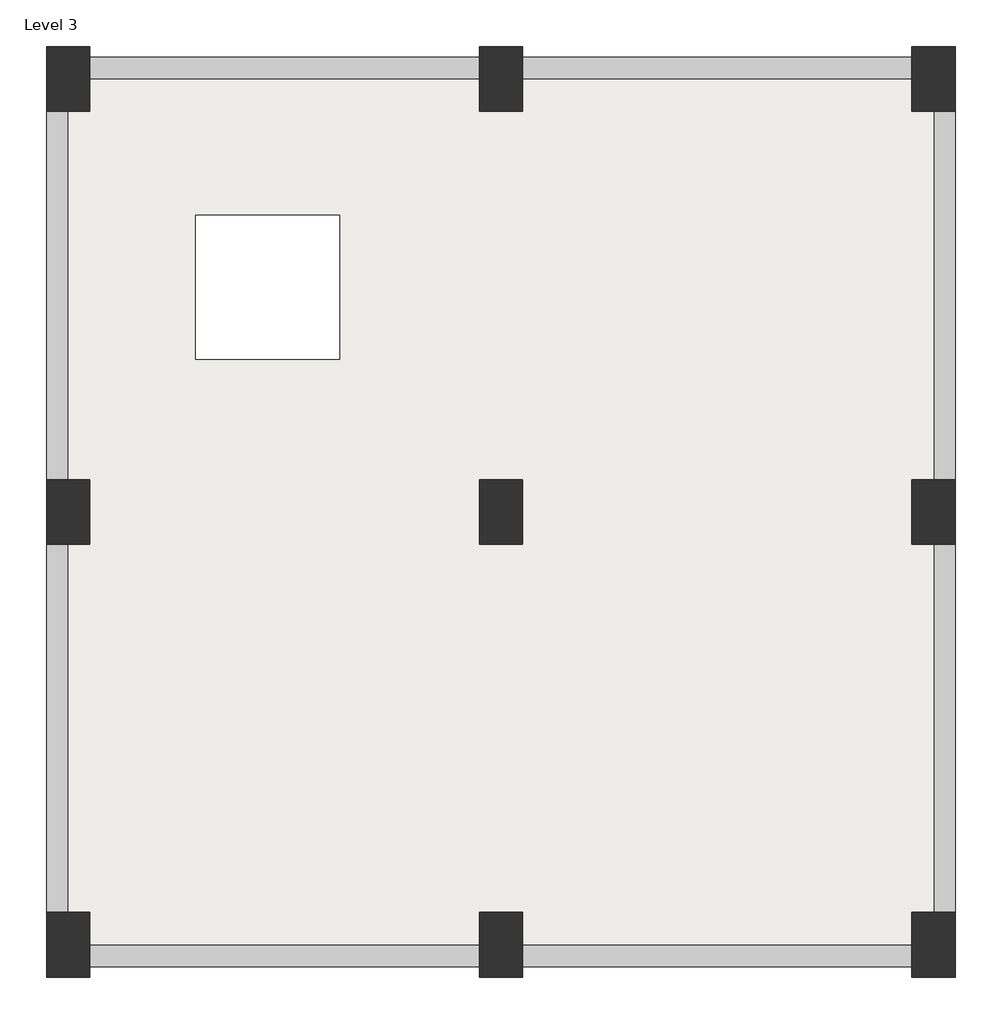
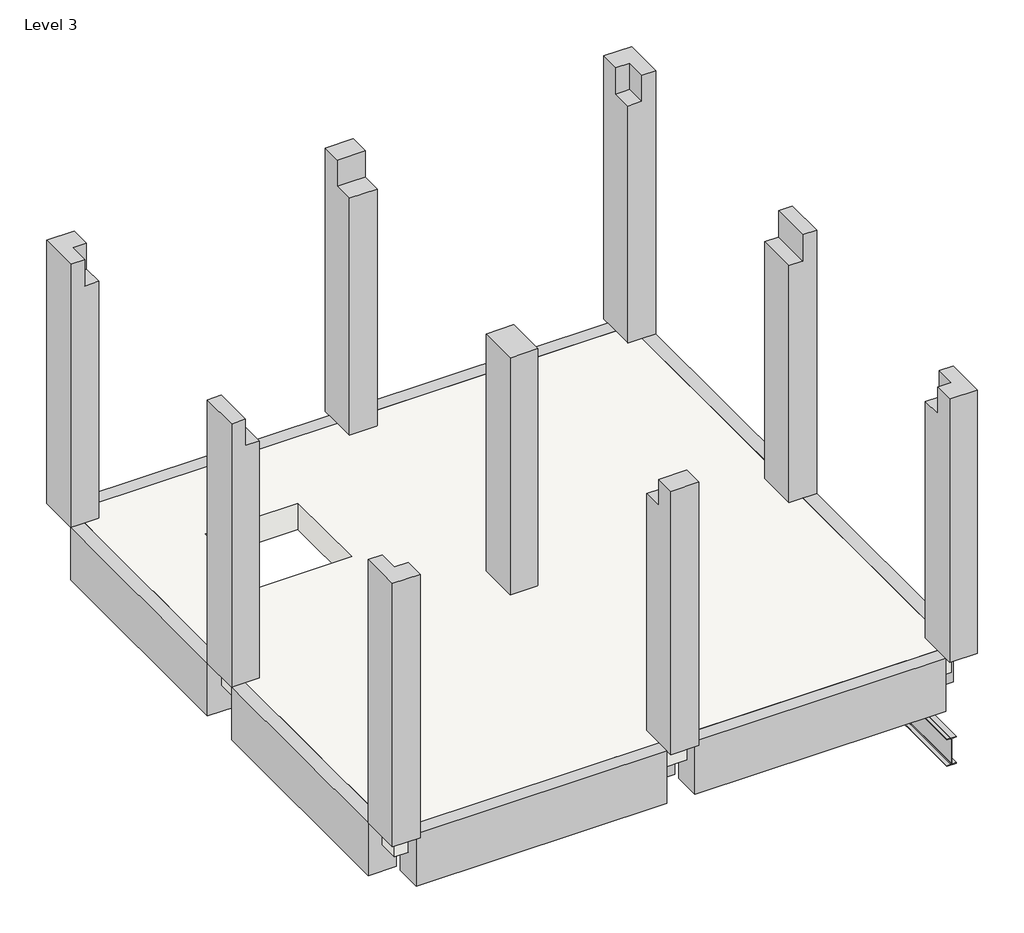
# One storey: 9 columns, 7 beams, 2 slabs.
"""IFC4 building model written with IfcOpenShell, lengths in millimetres."""

from ifc_helpers import new_model, si_unit, frame, origin, place, context, project, spatial, polyline, outline, extrude, faceted_brep, transform, mapped, element, save
from components import ub_universal_beams_ub305x102x25_07ba02ff

model = new_model("IFC4")

# Units and contexts
model_context = context("Model", 3, world=origin())
ifc_project = project(units=[si_unit("LENGTHUNIT", "METRE", prefix="MILLI")], contexts=[model_context])

# Site, building, storey
site = spatial("IfcSite", under=ifc_project)
building = spatial("IfcBuilding", under=site)
storey = spatial("IfcBuildingStorey", under=building, Name="Level 3", Elevation=6000.0)

# Beams
placement = place(None, origin())
element("IfcBeam", 1, ObjectType="Concrete-Rectangular Beam : 300 x 600mm", at=placement, inside=storey, context=model_context, shape_type="SweptSolid", body=[
    extrude(outline(polyline([(526.3372902, 5400.0), (226.3372902, 5400.0), (226.3372902, 5700.0), (376.3372902, 5700.0), (376.3372902, 6000.0), (526.3372902, 6000.0), (526.3372902, 5400.0)])), frame((2068.7595868, 0.0, 0.0), z_axis=(1.0, 0.0, 0.0), x_axis=(0.0, 1.0, 0.0)), (0.0, 0.0, 1.0), 2700.0),
    extrude(outline(polyline([(526.3372902, 5400.0), (226.3372902, 5400.0), (226.3372902, 5700.0), (376.3372902, 5700.0), (376.3372902, 6000.0), (526.3372902, 6000.0), (526.3372902, 5400.0)])), frame((-931.2404132, 0.0, 0.0), z_axis=(1.0, 0.0, 0.0), x_axis=(0.0, 1.0, 0.0)), (0.0, 0.0, 1.0), 2700.0),
])
element("IfcBeam", 2, ObjectType="Concrete-Rectangular Beam : 300 x 600mm", at=placement, inside=storey, context=model_context, shape_type="SweptSolid", body=[
    extrude(outline(polyline([(5400.0, 5068.7595868), (6000.0, 5068.7595868), (6000.0, 4918.7595868), (5700.0, 4918.7595868), (5700.0, 4768.7595868), (5400.0, 4768.7595868), (5400.0, 5068.7595868)])), frame((0.0, -2398.6627098, 0.0), z_axis=(0.0, 1.0, 0.0), x_axis=(0.0, 0.0, 1.0)), (0.0, 0.0, 1.0), 2550.0),
    extrude(outline(polyline([(5400.0, 5068.7595868), (6000.0, 5068.7595868), (6000.0, 4918.7595868), (5700.0, 4918.7595868), (5700.0, 4768.7595868), (5400.0, 4768.7595868), (5400.0, 5068.7595868)])), frame((0.0, -5398.6627098, 0.0), z_axis=(0.0, 1.0, 0.0), x_axis=(0.0, 0.0, 1.0)), (0.0, 0.0, 1.0), 2550.0),
])
element("IfcBeam", 3, ObjectType="Concrete-Rectangular Beam : 300 x 600mm", at=placement, inside=storey, context=model_context, shape_type="SweptSolid", body=[
    extrude(outline(polyline([(-5773.6627098, 5400.0), (-5773.6627098, 6000.0), (-5623.6627098, 6000.0), (-5623.6627098, 5700.0), (-5473.6627098, 5700.0), (-5473.6627098, 5400.0), (-5773.6627098, 5400.0)])), frame((2068.7595868, 0.0, 0.0), z_axis=(1.0, 0.0, 0.0), x_axis=(0.0, 1.0, 0.0)), (0.0, 0.0, 1.0), 2700.0),
    extrude(outline(polyline([(-5773.6627098, 5400.0), (-5773.6627098, 6000.0), (-5623.6627098, 6000.0), (-5623.6627098, 5700.0), (-5473.6627098, 5700.0), (-5473.6627098, 5400.0), (-5773.6627098, 5400.0)])), frame((-931.2404132, 0.0, 0.0), z_axis=(1.0, 0.0, 0.0), x_axis=(0.0, 1.0, 0.0)), (0.0, 0.0, 1.0), 2700.0),
])
element("IfcBeam", 4, ObjectType="Concrete-Rectangular Beam : 300 x 600mm", at=placement, inside=storey, context=model_context, shape_type="SweptSolid", body=[
    extrude(outline(polyline([(6000.0, -1231.2404132), (5400.0, -1231.2404132), (5400.0, -931.2404132), (5700.0, -931.2404132), (5700.0, -1081.2404132), (6000.0, -1081.2404132), (6000.0, -1231.2404132)])), frame((0.0, -5398.6627098, 0.0), z_axis=(0.0, 1.0, 0.0), x_axis=(0.0, 0.0, 1.0)), (0.0, 0.0, 1.0), 2550.0),
    extrude(outline(polyline([(6000.0, -1231.2404132), (5400.0, -1231.2404132), (5400.0, -931.2404132), (5700.0, -931.2404132), (5700.0, -1081.2404132), (6000.0, -1081.2404132), (6000.0, -1231.2404132)])), frame((0.0, -2398.6627098, 0.0), z_axis=(0.0, 1.0, 0.0), x_axis=(0.0, 0.0, 1.0)), (0.0, 0.0, 1.0), 2550.0),
])
element("IfcBeam", 5, ObjectType="Concrete-Rectangular Beam : 300 x 600mm", at=placement, inside=storey, context=model_context, shape_type="SweptSolid", body=[
    extrude(outline(polyline([(2068.7595868, -5398.6627098), (1768.7595868, -5398.6627098), (1768.7595868, -2848.6627098), (2068.7595868, -2848.6627098), (2068.7595868, -5398.6627098)])), frame((0.0, 0.0, 5400.0), z_axis=(0.0, 0.0, 1.0), x_axis=(1.0, 0.0, 0.0)), (0.0, 0.0, 1.0), 300.0),
    extrude(outline(polyline([(1768.7595868, 151.3372902), (2068.7595868, 151.3372902), (2068.7595868, -2398.6627098), (1768.7595868, -2398.6627098), (1768.7595868, 151.3372902)])), frame((0.0, 0.0, 5400.0), z_axis=(0.0, 0.0, 1.0), x_axis=(1.0, 0.0, 0.0)), (0.0, 0.0, 1.0), 300.0),
])
element("IfcBeam", 6, ObjectType="Concrete-Rectangular Beam : 300 x 600mm", at=placement, inside=storey, context=model_context, shape_type="SweptSolid", body=[
    extrude(outline(polyline([(4768.7595868, -2473.6627098), (4768.7595868, -2773.6627098), (2068.7595868, -2773.6627098), (2068.7595868, -2473.6627098), (4768.7595868, -2473.6627098)])), frame((0.0, 0.0, 5400.0), z_axis=(0.0, 0.0, 1.0), x_axis=(1.0, 0.0, 0.0)), (0.0, 0.0, 1.0), 300.0),
    extrude(outline(polyline([(-931.2404132, -2773.6627098), (-931.2404132, -2473.6627098), (1768.7595868, -2473.6627098), (1768.7595868, -2773.6627098), (-931.2404132, -2773.6627098)])), frame((0.0, 0.0, 5400.0), z_axis=(0.0, 0.0, 1.0), x_axis=(1.0, 0.0, 0.0)), (0.0, 0.0, 1.0), 300.0),
])
ub_universal_beams_ub305x102x25_shape = ub_universal_beams_ub305x102x25_07ba02ff(model_context)
element("IfcBeam", 7, ObjectType="UB-Universal Beams : UB305x102x25", at=placement, inside=storey, context=model_context, shape_type="MappedRepresentation", body=[
    mapped(ub_universal_beams_ub305x102x25_shape, transform((4918.7595868, -2623.6627098, 4800.0), x_axis=(0.0, 1.0, 0.0), y_axis=(-1.0, 0.0, 0.0), z_axis=(0.0, 0.0, 1.0))),
])

# Columns
element("IfcColumn", 8, ObjectType="Concrete-Rectangular-Column : 300 x 450mm", at=placement, inside=storey, context=model_context, shape_type="Brep", body=[
    faceted_brep([(-1231.2404132, -5848.6627098, 9000.0), (-931.2404132, -5848.6627098, 9000.0), (-931.2404132, -5623.6627098, 9000.0), (-1081.2404132, -5623.6627098, 9000.0), (-1081.2404132, -5398.6627098, 9000.0), (-1231.2404132, -5398.6627098, 9000.0), (-1231.2404132, -5848.6627098, 6000.0), (-1231.2404132, -5398.6627098, 6000.0), (-931.2404132, -5398.6627098, 6000.0), (-931.2404132, -5848.6627098, 6000.0), (-931.2404132, -5398.6627098, 8700.0), (-931.2404132, -5623.6627098, 8700.0), (-1081.2404132, -5398.6627098, 8700.0), (-1081.2404132, -5623.6627098, 8700.0)], [[[0, 1, 2, 3, 4, 5]], [[6, 7, 8, 9]], [[1, 0, 6, 9]], [[9, 8, 10, 11, 2, 1]], [[8, 7, 5, 4, 12, 10]], [[0, 5, 7, 6]], [[12, 13, 11, 10]], [[13, 3, 2, 11]], [[3, 13, 12, 4]]]),
])
element("IfcColumn", 9, ObjectType="Concrete-Rectangular-Column : 300 x 450mm", at=placement, inside=storey, context=model_context, shape_type="Brep", body=[
    faceted_brep([(1768.7595868, -5848.6627098, 9000.0), (2068.7595868, -5848.6627098, 9000.0), (2068.7595868, -5773.6627098, 9000.0), (2068.7595868, -5623.6627098, 9000.0), (1768.7595868, -5623.6627098, 9000.0), (1768.7595868, -5773.6627098, 9000.0), (1768.7595868, -5848.6627098, 6000.0), (1768.7595868, -5398.6627098, 6000.0), (2068.7595868, -5398.6627098, 6000.0), (2068.7595868, -5848.6627098, 6000.0), (2068.7595868, -5398.6627098, 8700.0), (2068.7595868, -5473.6627098, 8700.0), (2068.7595868, -5623.6627098, 8700.0), (1768.7595868, -5398.6627098, 8700.0), (1768.7595868, -5623.6627098, 8700.0), (1768.7595868, -5473.6627098, 8700.0)], [[[0, 1, 2, 3, 4, 5]], [[6, 7, 8, 9]], [[1, 0, 6, 9]], [[9, 8, 10, 11, 12, 3, 2, 1]], [[8, 7, 13, 10]], [[7, 6, 0, 5, 4, 14, 15, 13]], [[14, 12, 11, 10, 13, 15]], [[12, 14, 4, 3]]]),
])
element("IfcColumn", 10, ObjectType="Concrete-Rectangular-Column : 300 x 450mm", at=placement, inside=storey, context=model_context, shape_type="Brep", body=[
    faceted_brep([(4768.7595868, -5848.6627098, 9000.0), (5068.7595868, -5848.6627098, 9000.0), (5068.7595868, -5398.6627098, 9000.0), (4918.7595868, -5398.6627098, 9000.0), (4918.7595868, -5623.6627098, 9000.0), (4768.7595868, -5623.6627098, 9000.0), (4768.7595868, -5848.6627098, 6000.0), (4768.7595868, -5398.6627098, 6000.0), (5068.7595868, -5398.6627098, 6000.0), (5068.7595868, -5848.6627098, 6000.0), (4768.7595868, -5398.6627098, 8700.0), (4918.7595868, -5398.6627098, 8700.0), (4768.7595868, -5623.6627098, 8700.0), (4918.7595868, -5623.6627098, 8700.0)], [[[0, 1, 2, 3, 4, 5]], [[6, 7, 8, 9]], [[1, 0, 6, 9]], [[2, 1, 9, 8]], [[8, 7, 10, 11, 3, 2]], [[7, 6, 0, 5, 12, 10]], [[12, 13, 11, 10]], [[13, 4, 3, 11]], [[4, 13, 12, 5]]]),
])
element("IfcColumn", 11, ObjectType="Concrete-Rectangular-Column : 300 x 450mm", at=placement, inside=storey, context=model_context, shape_type="Brep", body=[
    faceted_brep([(-1231.2404132, -2398.6627098, 9000.0), (-1231.2404132, -2848.6627098, 9000.0), (-1081.2404132, -2848.6627098, 9000.0), (-1081.2404132, -2398.6627098, 9000.0), (-1231.2404132, -2848.6627098, 6000.0), (-1231.2404132, -2398.6627098, 6000.0), (-931.2404132, -2398.6627098, 6000.0), (-931.2404132, -2848.6627098, 6000.0), (-931.2404132, -2848.6627098, 8400.0), (-931.2404132, -2848.6627098, 8700.0), (-1081.2404132, -2848.6627098, 8700.0), (-1231.2404132, -2848.6627098, 8400.0), (-931.2404132, -2398.6627098, 8400.0), (-931.2404132, -2398.6627098, 8700.0), (-1231.2404132, -2398.6627098, 8400.0), (-1081.2404132, -2398.6627098, 8700.0)], [[[0, 1, 2, 3]], [[4, 5, 6, 7]], [[4, 7, 8, 9, 10, 2, 1, 11]], [[7, 6, 12, 13, 9, 8]], [[6, 5, 14, 0, 3, 15, 13, 12]], [[1, 0, 14, 5, 4, 11]], [[15, 10, 9, 13]], [[10, 15, 3, 2]]]),
])
element("IfcColumn", 12, ObjectType="Concrete-Rectangular-Column : 300 x 450mm", at=placement, inside=storey, context=model_context, shape_type="Brep", body=[
    faceted_brep([(1768.7595868, -2848.6627098, 6000.0), (1768.7595868, -2398.6627098, 6000.0), (2068.7595868, -2398.6627098, 6000.0), (2068.7595868, -2848.6627098, 6000.0), (2068.7595868, -2848.6627098, 8700.0), (1768.7595868, -2848.6627098, 8700.0), (2068.7595868, -2398.6627098, 8700.0), (2068.7595868, -2473.6627098, 8700.0), (2068.7595868, -2773.6627098, 8700.0), (1768.7595868, -2398.6627098, 8700.0), (1768.7595868, -2773.6627098, 8700.0), (1768.7595868, -2473.6627098, 8700.0)], [[[0, 1, 2, 3]], [[0, 3, 4, 5]], [[3, 2, 6, 7, 8, 4]], [[2, 1, 9, 6]], [[1, 0, 5, 10, 11, 9]], [[5, 4, 8, 7, 6, 9, 11, 10]]]),
])
element("IfcColumn", 13, ObjectType="Concrete-Rectangular-Column : 300 x 450mm", at=placement, inside=storey, context=model_context, shape_type="SweptSolid", body=[
    extrude(outline(polyline([(6000.0, 4768.7595868), (6000.0, 5068.7595868), (9000.0, 5068.7595868), (9000.0, 4918.7595868), (8700.0, 4918.7595868), (8700.0, 4768.7595868), (6000.0, 4768.7595868)])), frame((0.0, -2848.6627098, 0.0), z_axis=(0.0, 1.0, 0.0), x_axis=(0.0, 0.0, 1.0)), (0.0, 0.0, 1.0), 450.0),
])
element("IfcColumn", 14, ObjectType="Concrete-Rectangular-Column : 300 x 450mm", at=placement, inside=storey, context=model_context, shape_type="Brep", body=[
    faceted_brep([(-931.2404132, 601.3372902, 9000.0), (-1231.2404132, 601.3372902, 9000.0), (-1231.2404132, 151.3372902, 9000.0), (-1081.2404132, 151.3372902, 9000.0), (-1081.2404132, 376.3372902, 9000.0), (-931.2404132, 376.3372902, 9000.0), (-1231.2404132, 151.3372902, 6000.0), (-1231.2404132, 601.3372902, 6000.0), (-931.2404132, 601.3372902, 6000.0), (-931.2404132, 151.3372902, 6000.0), (-931.2404132, 151.3372902, 8700.0), (-1081.2404132, 151.3372902, 8700.0), (-931.2404132, 376.3372902, 8700.0), (-1081.2404132, 376.3372902, 8700.0)], [[[0, 1, 2, 3, 4, 5]], [[6, 7, 8, 9]], [[6, 9, 10, 11, 3, 2]], [[9, 8, 0, 5, 12, 10]], [[1, 0, 8, 7]], [[2, 1, 7, 6]], [[12, 13, 11, 10]], [[13, 4, 3, 11]], [[4, 13, 12, 5]]]),
])
element("IfcColumn", 15, ObjectType="Concrete-Rectangular-Column : 300 x 450mm", at=placement, inside=storey, context=model_context, shape_type="Brep", body=[
    faceted_brep([(2068.7595868, 601.3372902, 9000.0), (1768.7595868, 601.3372902, 9000.0), (1768.7595868, 526.3372902, 9000.0), (1768.7595868, 376.3372902, 9000.0), (2068.7595868, 376.3372902, 9000.0), (2068.7595868, 526.3372902, 9000.0), (1768.7595868, 151.3372902, 6000.0), (1768.7595868, 601.3372902, 6000.0), (2068.7595868, 601.3372902, 6000.0), (2068.7595868, 151.3372902, 6000.0), (2068.7595868, 151.3372902, 8700.0), (1768.7595868, 151.3372902, 8700.0), (2068.7595868, 376.3372902, 8700.0), (2068.7595868, 226.3372902, 8700.0), (1768.7595868, 226.3372902, 8700.0), (1768.7595868, 376.3372902, 8700.0)], [[[0, 1, 2, 3, 4, 5]], [[6, 7, 8, 9]], [[6, 9, 10, 11]], [[9, 8, 0, 5, 4, 12, 13, 10]], [[1, 0, 8, 7]], [[7, 6, 11, 14, 15, 3, 2, 1]], [[12, 15, 14, 11, 10, 13]], [[15, 12, 4, 3]]]),
])
element("IfcColumn", 16, ObjectType="Concrete-Rectangular-Column : 300 x 450mm", at=placement, inside=storey, context=model_context, shape_type="Brep", body=[
    faceted_brep([(5068.7595868, 151.3372902, 9000.0), (5068.7595868, 601.3372902, 9000.0), (4768.7595868, 601.3372902, 9000.0), (4768.7595868, 376.3372902, 9000.0), (4918.7595868, 376.3372902, 9000.0), (4918.7595868, 151.3372902, 9000.0), (4768.7595868, 151.3372902, 6000.0), (4768.7595868, 601.3372902, 6000.0), (5068.7595868, 601.3372902, 6000.0), (5068.7595868, 151.3372902, 6000.0), (4918.7595868, 151.3372902, 8700.0), (4768.7595868, 151.3372902, 8700.0), (4768.7595868, 376.3372902, 8700.0), (4918.7595868, 376.3372902, 8700.0)], [[[0, 1, 2, 3, 4, 5]], [[6, 7, 8, 9]], [[6, 9, 0, 5, 10, 11]], [[1, 0, 9, 8]], [[2, 1, 8, 7]], [[7, 6, 11, 12, 3, 2]], [[13, 12, 11, 10]], [[4, 13, 10, 5]], [[13, 4, 3, 12]]]),
])

# Slabs
element("IfcSlab", 17, ObjectType="Generic 300mm", at=placement, inside=storey, context=model_context, shape_type="Brep", body=[
    faceted_brep([(4918.7595868, 376.3372902, 5700.0), (4918.7595868, 151.3372902, 5700.0), (4918.7595868, -2398.6627098, 5700.0), (4918.7595868, -2848.6627098, 5700.0), (4918.7595868, -5398.6627098, 5700.0), (4918.7595868, -5623.6627098, 5700.0), (4768.7595868, -5623.6627098, 5700.0), (2068.7595868, -5623.6627098, 5700.0), (1768.7595868, -5623.6627098, 5700.0), (-931.2404132, -5623.6627098, 5700.0), (-1081.2404132, -5623.6627098, 5700.0), (-1081.2404132, -5398.6627098, 5700.0), (-1081.2404132, -2848.6627098, 5700.0), (-1081.2404132, -2398.6627098, 5700.0), (-1081.2404132, 151.3372902, 5700.0), (-1081.2404132, 376.3372902, 5700.0), (-931.2404132, 376.3372902, 5700.0), (1768.7595868, 376.3372902, 5700.0), (2068.7595868, 376.3372902, 5700.0), (4768.7595868, 376.3372902, 5700.0), (-198.5229478, -1566.5574371, 5700.0), (801.4770522, -1566.5574371, 5700.0), (801.4770522, -566.5574371, 5700.0), (-198.5229478, -566.5574371, 5700.0), (4918.7595868, -5623.6627098, 6000.0), (4918.7595868, -5398.6627098, 6000.0), (4918.7595868, -2848.6627098, 6000.0), (4918.7595868, -2398.6627098, 6000.0), (4918.7595868, 151.3372902, 6000.0), (4918.7595868, 376.3372902, 6000.0), (4768.7595868, 376.3372902, 6000.0), (2068.7595868, 376.3372902, 6000.0), (1768.7595868, 376.3372902, 6000.0), (-931.2404132, 376.3372902, 6000.0), (-1081.2404132, 376.3372902, 6000.0), (-1081.2404132, 151.3372902, 6000.0), (-1081.2404132, -2398.6627098, 6000.0), (-1081.2404132, -2848.6627098, 6000.0), (-1081.2404132, -5398.6627098, 6000.0), (-1081.2404132, -5623.6627098, 6000.0), (-931.2404132, -5623.6627098, 6000.0), (1768.7595868, -5623.6627098, 6000.0), (2068.7595868, -5623.6627098, 6000.0), (4768.7595868, -5623.6627098, 6000.0), (801.4770522, -1566.5574371, 6000.0), (-198.5229478, -1566.5574371, 6000.0), (-198.5229478, -566.5574371, 6000.0), (801.4770522, -566.5574371, 6000.0)], [[[0, 1, 2, 3, 4, 5, 6, 7, 8, 9, 10, 11, 12, 13, 14, 15, 16, 17, 18, 19], [20, 21, 22, 23]], [[24, 25, 26, 27, 28, 29, 30, 31, 32, 33, 34, 35, 36, 37, 38, 39, 40, 41, 42, 43], [44, 45, 46, 47]], [[5, 4, 3, 2, 1, 0, 29, 28, 27, 26, 25, 24]], [[10, 9, 8, 7, 6, 5, 24, 43, 42, 41, 40, 39]], [[15, 14, 13, 12, 11, 10, 39, 38, 37, 36, 35, 34]], [[0, 19, 18, 17, 16, 15, 34, 33, 32, 31, 30, 29]], [[20, 45, 44, 21]], [[21, 44, 47, 22]], [[22, 47, 46, 23]], [[45, 20, 23, 46]]]),
])
element("IfcSlab", 18, ObjectType="Generic 300mm", at=placement, inside=storey, context=model_context, shape_type="Brep", body=[
    faceted_brep([(4918.7595868, 376.3372902, 5700.0), (4918.7595868, 151.3372902, 5700.0), (4918.7595868, -2398.6627098, 5700.0), (4918.7595868, -2848.6627098, 5700.0), (4918.7595868, -5398.6627098, 5700.0), (4918.7595868, -5623.6627098, 5700.0), (4768.7595868, -5623.6627098, 5700.0), (2068.7595868, -5623.6627098, 5700.0), (1768.7595868, -5623.6627098, 5700.0), (-931.2404132, -5623.6627098, 5700.0), (-1081.2404132, -5623.6627098, 5700.0), (-1081.2404132, -5398.6627098, 5700.0), (-1081.2404132, -2848.6627098, 5700.0), (-1081.2404132, -2398.6627098, 5700.0), (-1081.2404132, 151.3372902, 5700.0), (-1081.2404132, 376.3372902, 5700.0), (-931.2404132, 376.3372902, 5700.0), (1768.7595868, 376.3372902, 5700.0), (2068.7595868, 376.3372902, 5700.0), (4768.7595868, 376.3372902, 5700.0), (-198.5229478, -1566.5574371, 5700.0), (801.4770522, -1566.5574371, 5700.0), (801.4770522, -566.5574371, 5700.0), (-198.5229478, -566.5574371, 5700.0), (4918.7595868, -5623.6627098, 6000.0), (4918.7595868, -5398.6627098, 6000.0), (4918.7595868, -2848.6627098, 6000.0), (4918.7595868, -2398.6627098, 6000.0), (4918.7595868, 151.3372902, 6000.0), (4918.7595868, 376.3372902, 6000.0), (4768.7595868, 376.3372902, 6000.0), (2068.7595868, 376.3372902, 6000.0), (1768.7595868, 376.3372902, 6000.0), (-931.2404132, 376.3372902, 6000.0), (-1081.2404132, 376.3372902, 6000.0), (-1081.2404132, 151.3372902, 6000.0), (-1081.2404132, -2398.6627098, 6000.0), (-1081.2404132, -2848.6627098, 6000.0), (-1081.2404132, -5398.6627098, 6000.0), (-1081.2404132, -5623.6627098, 6000.0), (-931.2404132, -5623.6627098, 6000.0), (1768.7595868, -5623.6627098, 6000.0), (2068.7595868, -5623.6627098, 6000.0), (4768.7595868, -5623.6627098, 6000.0), (801.4770522, -1566.5574371, 6000.0), (-198.5229478, -1566.5574371, 6000.0), (-198.5229478, -566.5574371, 6000.0), (801.4770522, -566.5574371, 6000.0)], [[[0, 1, 2, 3, 4, 5, 6, 7, 8, 9, 10, 11, 12, 13, 14, 15, 16, 17, 18, 19], [20, 21, 22, 23]], [[24, 25, 26, 27, 28, 29, 30, 31, 32, 33, 34, 35, 36, 37, 38, 39, 40, 41, 42, 43], [44, 45, 46, 47]], [[5, 4, 3, 2, 1, 0, 29, 28, 27, 26, 25, 24]], [[10, 9, 8, 7, 6, 5, 24, 43, 42, 41, 40, 39]], [[15, 14, 13, 12, 11, 10, 39, 38, 37, 36, 35, 34]], [[0, 19, 18, 17, 16, 15, 34, 33, 32, 31, 30, 29]], [[20, 45, 44, 21]], [[21, 44, 47, 22]], [[22, 47, 46, 23]], [[45, 20, 23, 46]]]),
])

save(model, "model.ifc")

# Revit data of these elements
# Type "Concrete-Rectangular Beam : 300 x 600mm"
#   Length [instance default] = 1.524 m
#   b = 0.3 m
#   h = 0.6 m
#   Structural Material [instance default] = Concrete, Cast-in-Place gray
#   Assembly Code = ""
# Type "UB-Universal Beams : UB305x102x25"
#   Section Name Key = "UB305X102X25"
#   Width = 10.16 cm
#   Web Thickness = 0.58 cm
#   Web Fillet = 0.76 cm
#   Warping Constant = 27300.0 cm⁶
#   Torsional Moment of Inertia = 4.77 cm⁴
#   Section Area = 31.6 cm²
#   Plastic Modulus weak axis = 39.0 cm³
#   Plastic Modulus strong axis = 342.0 cm³
#   Nominal Weight = 24.7999 kgf/m
#   Moment of Inertia weak axis = 123.00 cm⁴
#   Moment of Inertia strong axis = 4455.00 cm⁴
#   Height = 30.51 cm
#   Flange Thickness = 0.7 cm
#   Elastic Modulus weak axis = 24.2 cm³
#   Elastic Modulus strong axis = 292.0 cm³
#   Centroid Vertical = 15.255 cm
#   Centroid Horizontal = 5.08 cm
#   Bolt Spacing = 5.4 cm
#   Length [instance default] = 1.5 m
#   Structural Material [instance default] = Metal - Steel 43-275
#   Type Comments = ""
#   Assembly Code = ""
# Type "Concrete-Rectangular-Column : 300 x 450mm"
#   b = 0.3 m
#   h = 0.45 m
#   Structural Material [instance default] = Concrete, Cast-in-Place gray
# Type "Generic 300mm"
#   Function = 0
#   Layers, outside or top first: 0.3 m no material (function 1)
# Elements 1, 2, 3, 4, 5, 6 (IfcBeam, "Concrete-Rectangular Beam : 300 x 600mm")
#   Structural Material = Concrete, Cast-in-Place gray
#   Phase Created = New Construction
#   Materials on its faces: "Concrete, Cast-in-Place gray"
# Element 7 (IfcBeam, "UB-Universal Beams : UB305x102x25")
#   Structural Material = Metal - Steel 43-275
#   Phase Created = New Construction
#   Materials on its faces: "Metal - Steel 43-275"
# Elements 8, 9, 10, 11, 12, 13, 14, 15, 16 (IfcColumn, "Concrete-Rectangular-Column : 300 x 450mm")
#   Structural Material = Concrete, Cast-in-Place gray
#   Phase Created = New Construction
#   Materials on its faces: "Concrete, Cast-in-Place gray"
# Elements 17, 18 (IfcSlab, "Generic 300mm")
#   Height Offset From Level = 0 m
#   built-in parameter 1001954 = 1
#   Phase Created = New Construction
#   Materials on its faces: "Default Floor"
# Materials
#   "Concrete, Cast-in-Place gray": class "Concrete", colour RGB 192 192 192, transparency 0, Description = "Cast-in-place concrete", Cost = 0
#   "Metal - Steel 43-275": class "Metal", colour RGB 247 247 247, transparency 0, Cost = 0
#   "Default Floor": colour RGB 127 127 127, transparency 0, Cost = 0
